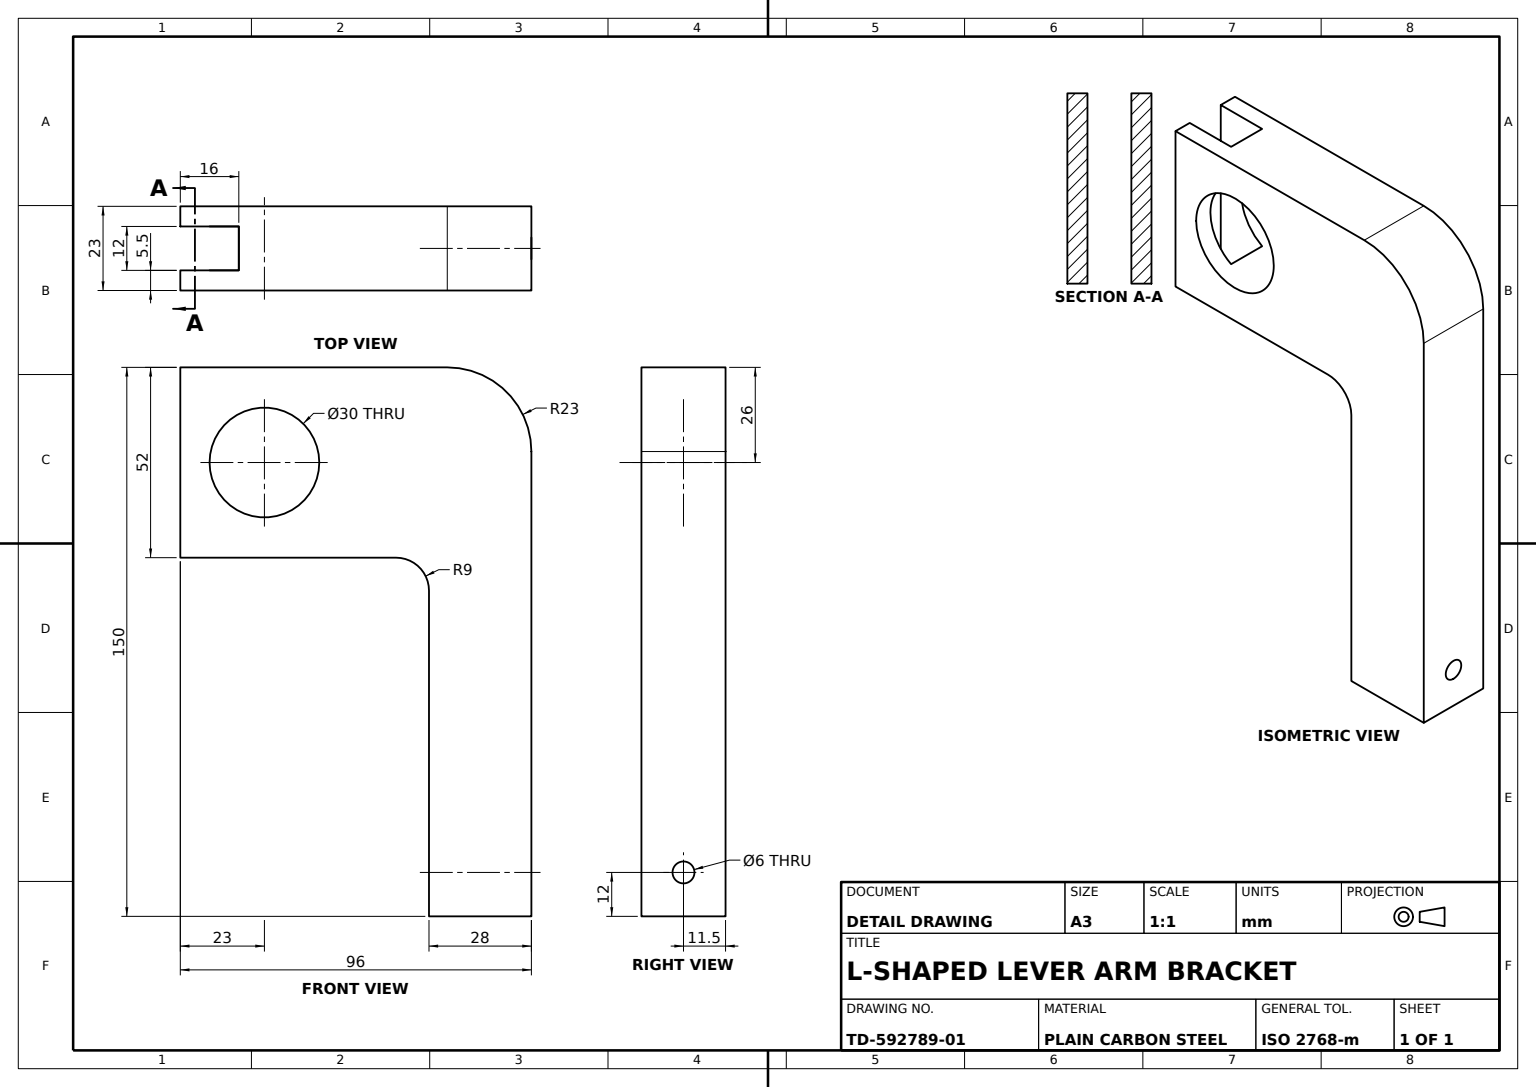
from build123d import *

# Parameters (mm, degrees)
BRACKET_PROFILE_SKETCH_R = 15
L_BRACKET_BODY_DEPTH     = 11.5
SLOT_CUT_SKETCH_W        = 16
SLOT_CUT_SKETCH_H        = 12
SLOT_CUT_DEPTH           = 63
END_HOLE_SKETCH_R        = 3
END_HOLE_DEPTH           = 63


with BuildPart() as part:
    # Bracket Profile Sketch → L-Bracket Body (new, symmetric)
    with BuildSketch(Plane.XY):
        with BuildLine():
            Line((73, 3), (73, -124))
            Line((73, -124), (45, -124))
            Line((45, -124), (45, -35))
            ThreePointArc((45, -35), (42.363961031, -28.636038969), (36, -26))
            Line((36, -26), (-23, -26))
            Line((-23, -26), (-23, 26))
            Line((-23, 26), (50, 26))
            ThreePointArc((50, 26), (66.263455967, 19.263455967), (73, 3))
        make_face()
        Circle(BRACKET_PROFILE_SKETCH_R, mode=Mode.SUBTRACT)
    extrude(amount=L_BRACKET_BODY_DEPTH, both=True)

    # Slot Cut Sketch → Slot Cut (cut)
    with BuildSketch(Plane(origin=(0, 26, 0), x_dir=(1, 0, 0), z_dir=(0, 1, 0))):
        with Locations((-15, 0)):
            Rectangle(SLOT_CUT_SKETCH_W, SLOT_CUT_SKETCH_H)
    extrude(amount=-SLOT_CUT_DEPTH, mode=Mode.SUBTRACT)

    # End Hole Sketch → End Hole (cut)
    with BuildSketch(Plane(origin=(73, 0, 0), x_dir=(0, 0, -1), z_dir=(1, 0, 0))):
        with Locations(Location((0, -112, 0), (0, 0, 90))):
            Circle(END_HOLE_SKETCH_R)
    extrude(amount=-END_HOLE_DEPTH, mode=Mode.SUBTRACT)


solid = part.part
